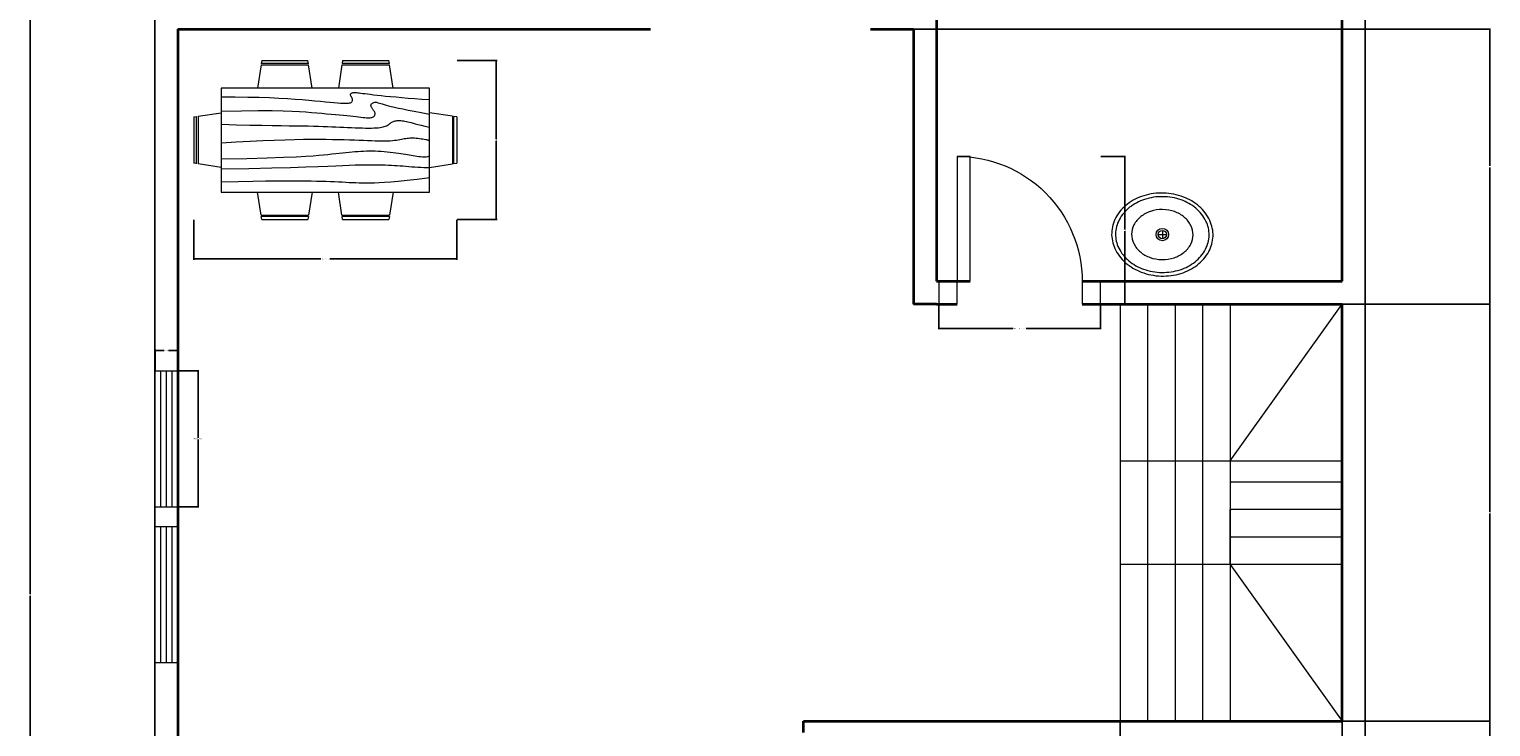
# Model space of a CAD drawing. Units: feet. Extents: x 2306 to 3052, y 829 to 1424.
# Tile 2 of 5: x 2306 to 2625, y 1098 to 1250. Entities that reach past the tile are written whole.
import ezdxf

# ---------------------------------------------------------------- set-up
doc = ezdxf.new("R2010")
doc.units = ezdxf.units.FT
for name, color, linetype, lineweight in [('A-ANNO-DIMS', 2, 'Continuous', 18), ('A-DOOR', 3, 'Continuous', 18), ('A-FLOR-FIXT', 9, 'Continuous', 18), ('A-FLOR-OTLN', 7, 'Continuous', 25), ('A-FLOR-STRS', 7, 'Continuous', 18), ('A-FURN', 8, 'Continuous', 13), ('A-GLAZ', 4, 'Continuous', 18), ('A-WALL', 7, 'Continuous', 35)]:
    doc.layers.add(name, color=color, linetype=linetype, lineweight=lineweight)
doc.styles.get("Standard").update_dxf_attribs({"font": 'arial.ttf'})
doc.dimstyles.get("Standard").update_dxf_attribs({"dimtxt": 0.18, "dimasz": 0.18, "dimexe": 0.18, "dimexo": 0.0625, "dimgap": 0.09, "dimtad": 0, "dimtih": 1, "dimtoh": 1, "dimdec": 4, "dimzin": 0, "dimdsep": 46, "dimlunit": 4, "dimtxsty": 'Standard', "dimcen": 0.09, "dimadec": 0, "dimazin": 0, "dimtfac": 1, "dimtdec": 4, "dimtofl": 0, "dimtmove": 0, "dimatfit": 3, "dimfxl": 1, "dimtolj": 1, "dimtzin": 0, "dimarcsym": 0})

# ---------------------------------------------------------------- blocks, each defined once
blk = doc.blocks.new('Window - Wood Frame 36 in. Wide plan')
for p, q in [((0, 6), (0, 0)), ((0, 4.5), (36, 4.5)), ((36, 6), (36, 0)), ((0, 3), (36, 3)), ((0, 1.5), (36, 1.5))]:
    blk.add_line(p, q)
blk = doc.blocks.new('Dining Set - 36 x 72 in.')
for p, q in [((-22.2343, 26.00059), (-23.4847, 17.99762)), ((-22.2304, 26), (-5.7608, 26)), ((-22, 27.5), (-22.1562, 26.50042)), ((-5.8416, 26.5), (-22.1534, 26.5)), ((-22, 27.5), (-6, 27.5)), ((-5.8437, 26.49966), (-6, 27.5)), ((-4.5152, 17.99762), (-5.7655, 25.99926)), ((5.7657, 26.00059), (4.5153, 17.99762)), ((5.7696, 26), (22.2392, 26)), ((6, 27.5), (5.8438, 26.50042)), ((22.1584, 26.5), (5.8466, 26.5)), ((6, 27.5), (22, 27.5)), ((22.1563, 26.49966), (22, 27.5)), ((23.4848, 17.99762), (22.2345, 25.99926)), ((36, 18), (-36, 18)), ((-36, 18), (-36, -18)), ((36, -18), (36, 18)), ((-45.5, 8), (-44.5004, 8.15617)), ((-45.5, 8), (-45.5, -8)), ((-44.5, -8.15843), (-44.5, 8.15338)), ((-44.0006, 8.23428), (-35.9976, 9.48474)), ((-44, 8.23041), (-44, -8.23915)), ((44.0006, 8.23428), (35.9976, 9.48474)), ((44, 8.23041), (44, -8.23915)), ((44.5, -8.15843), (44.5, 8.15338)), ((45.5, 8), (44.5005, 8.15617)), ((45.5, 8), (45.5, -8)), ((-44.4997, -8.15631), (-45.5, -8)), ((-35.9976, -9.48476), (-43.9993, -8.2345)), ((35.9976, -9.48476), (43.9993, -8.2345)), ((44.4997, -8.15631), (45.5, -8)), ((-36, -18), (36, -18)), ((-22.2343, -26.0006), (-23.4847, -17.99762)), ((-4.5152, -17.99762), (-5.7655, -25.99928)), ((5.7657, -26.0006), (4.5153, -17.99762)), ((23.4848, -17.99762), (22.2345, -25.99928)), ((-22.2304, -26), (-5.7608, -26)), ((-22, -27.5), (-22.1562, -26.50044)), ((-5.8416, -26.5), (-22.1534, -26.5)), ((-22, -27.5), (-6, -27.5)), ((-5.8437, -26.49967), (-6, -27.5)), ((5.7696, -26), (22.2392, -26)), ((6, -27.5), (5.8438, -26.50044)), ((22.1584, -26.5), (5.8466, -26.5)), ((6, -27.5), (22, -27.5)), ((22.1563, -26.49967), (22, -27.5))]:
    blk.add_line(p, q)
for points in [[(-36, 15), (-31.1772, 14.97754), (-26.8079, 14.91406), (-22.8538, 14.81543), (-19.276, 14.6875), (-16.0362, 14.53613), (-13.0957, 14.36718), (-10.4159, 14.18652), (-7.9583, 14), (-5.6904, 13.81315), (-3.6035, 13.63021), (-1.6954, 13.45508), (0.0365, 13.29166), (1.5945, 13.14388), (2.9811, 13.01562), (4.1988, 12.9108), (5.25, 12.83333), (6.1393, 12.78613), (6.8802, 12.76823), (7.4883, 12.77767), (7.9792, 12.8125), (8.3685, 12.87077), (8.6719, 12.95052), (8.9049, 13.0498), (9.0833, 13.16666), (9.2205, 13.29899), (9.3216, 13.44401), (9.3895, 13.59879), (9.4271, 13.76041), (9.4373, 13.92594), (9.4232, 14.09245), (9.3875, 14.257), (9.3333, 14.41666), (9.2638, 14.56917), (9.1836, 14.71484), (9.0975, 14.85465), (9.0104, 14.98958), (8.9272, 15.1206), (8.8529, 15.2487), (8.7922, 15.37483), (8.75, 15.5), (8.7305, 15.62467), (8.7344, 15.74739), (8.7617, 15.86621), (8.8125, 15.97916), (8.8867, 16.08431), (8.9844, 16.17968), (9.1055, 16.26334), (9.25, 16.33333), (9.4189, 16.38802), (9.6172, 16.42708), (9.8506, 16.45052), (10.125, 16.45833), (10.4463, 16.45052), (10.8203, 16.42708), (11.2529, 16.38802), (11.75, 16.33333), (12.3184, 16.26318), (12.9694, 16.17838), (13.7151, 16.07991), (14.5677, 15.96875), (15.5395, 15.84586), (16.6426, 15.71224), (17.8893, 15.56884), (19.2917, 15.41666), (20.859, 15.25667), (22.5879, 15.08984), (24.4721, 14.91715), (26.5052, 14.73958), (28.6809, 14.5581), (30.9929, 14.3737), (33.4347, 14.18733), (36, 14)], [(-36, 10), (-28.9766, 10.14274), (-23.1725, 10.20442), (-18.4241, 10.19775), (-14.5677, 10.13541), (-11.4399, 10.03011), (-8.877, 9.89453), (-6.7154, 9.74137), (-4.7917, 9.58333), (-2.9698, 9.43082), (-1.2246, 9.28515), (0.4415, 9.14534), (2.026, 9.01041), (3.5266, 8.87939), (4.9408, 8.7513), (6.266, 8.62516), (7.5, 8.5), (8.6411, 8.37549), (9.6914, 8.2539), (10.6538, 8.13818), (11.5312, 8.03125), (12.3267, 7.93603), (13.043, 7.85547), (13.6831, 7.79248), (14.25, 7.75), (14.7471, 7.7303), (15.1797, 7.73307), (15.5537, 7.75732), (15.875, 7.80208), (16.1494, 7.86637), (16.3828, 7.94922), (16.5811, 8.04964), (16.75, 8.16666), (16.8944, 8.29915), (17.0143, 8.44531), (17.1089, 8.60319), (17.1771, 8.77083), (17.218, 8.94629), (17.2305, 9.1276), (17.2137, 9.31282), (17.1667, 9.5), (17.0895, 9.6875), (16.987, 9.875), (16.8649, 10.0625), (16.7292, 10.25), (16.5856, 10.4375), (16.4401, 10.625), (16.2985, 10.8125), (16.1667, 11), (16.05, 11.18733), (15.9518, 11.3737), (15.8752, 11.5581), (15.8229, 11.73958), (15.798, 11.91715), (15.8034, 12.08984), (15.842, 12.25667), (15.9167, 12.41666), (16.0295, 12.56836), (16.1784, 12.70833), (16.3605, 12.83268), (16.5729, 12.9375), (16.8127, 13.01888), (17.0768, 13.07291), (17.3625, 13.0957), (17.6667, 13.08333), (17.9894, 13.03312), (18.3418, 12.94726), (18.7382, 12.82918), (19.1927, 12.68229), (19.7195, 12.51001), (20.3327, 12.31575), (21.0465, 12.10294), (21.875, 11.875), (22.8357, 11.63354), (23.959, 11.37304), (25.2786, 11.08618), (26.8282, 10.76562), (28.6414, 10.40405), (30.752, 9.99414), (33.1936, 9.52856), (36, 9)], [(-36, 5.5), (-30.7157, 5.3348), (-26.069, 5.20963), (-21.9946, 5.11767), (-18.4271, 5.05208), (-15.3009, 5.00602), (-12.5508, 4.97265), (-10.1112, 4.94515), (-7.9167, 4.91666), (-5.909, 4.88167), (-4.0586, 4.83984), (-2.3429, 4.79215), (-0.7396, 4.73958), (0.7739, 4.6831), (2.22, 4.6237), (3.6213, 4.56233), (5, 4.5), (6.373, 4.43782), (7.7344, 4.3776), (9.0723, 4.32129), (10.375, 4.27083), (11.6309, 4.22819), (12.8281, 4.19531), (13.9551, 4.17415), (15, 4.16666), (15.954, 4.17448), (16.819, 4.19791), (17.6001, 4.23698), (18.3021, 4.29166), (18.9299, 4.36198), (19.4883, 4.44791), (19.9823, 4.54948), (20.4167, 4.66666), (20.7969, 4.79899), (21.1302, 4.94401), (21.4245, 5.09879), (21.6875, 5.26041), (21.9271, 5.42594), (22.1511, 5.59245), (22.3672, 5.757), (22.5834, 5.91666), (22.8065, 6.06868), (23.0404, 6.21093), (23.2879, 6.34147), (23.5521, 6.45833), (23.8358, 6.55957), (24.142, 6.64323), (24.4735, 6.70735), (24.8334, 6.75), (25.2235, 6.76969), (25.642, 6.76692), (26.0858, 6.74267), (26.5521, 6.69791), (27.0379, 6.63362), (27.5404, 6.55078), (28.0565, 6.45036), (28.5834, 6.33333), (29.1242, 6.19987), (29.7071, 6.04687), (30.3661, 5.87044), (31.1354, 5.66666), (32.0493, 5.43164), (33.142, 5.16146), (34.4475, 4.85221), (36, 4.5)], [(-36, -1), (-30.7915, -0.6591), (-26.0195, -0.38216), (-21.6519, -0.16284), (-17.6563, 0.00521), (-14.0005, 0.12833), (-10.6523, 0.21289), (-7.5796, 0.26522), (-4.75, 0.29166), (-2.134, 0.29793), (0.2878, 0.28711), (2.5317, 0.26163), (4.6146, 0.22396), (6.5529, 0.17651), (8.3633, 0.12174), (10.0623, 0.06209), (11.6667, 0), (13.1899, -0.06201), (14.6341, -0.1211), (15.9982, -0.17432), (17.2813, -0.21875), (18.4823, -0.25147), (19.6003, -0.26953), (20.6343, -0.27002), (21.5834, -0.25), (22.4481, -0.20768), (23.2357, -0.14584), (23.9549, -0.06836), (24.6146, 0.02083), (25.2235, 0.11784), (25.7904, 0.21875), (26.3241, 0.31966), (26.8334, 0.41666), (27.3265, 0.50618), (27.8099, 0.58593), (28.2894, 0.65397), (28.7709, 0.70833), (29.2601, 0.74707), (29.763, 0.76823), (30.2855, 0.76985), (30.8334, 0.75), (31.4088, 0.70784), (31.9994, 0.64713), (32.589, 0.57275), (33.1615, 0.48958), (33.7008, 0.4025), (34.1908, 0.3164), (34.6153, 0.23616), (34.9584, 0.16666), (35.2099, 0.11165), (35.3848, 0.07031), (35.504, 0.04069), (35.5886, 0.02083), (35.6594, 0.00879), (35.7377, 0.0026), (35.8442, 0.00032), (36, 0)], [(-36, -6.5), (-27.1843, -6.31267), (-20.084, -6.1263), (-14.469, -5.9419), (-10.1094, -5.76042), (-6.7752, -5.58285), (-4.2363, -5.41016), (-2.2629, -5.24333), (-0.625, -5.08334), (0.8708, -4.93099), (2.2715, -4.78646), (3.5872, -4.64974), (4.8281, -4.52084), (6.0046, -4.39974), (7.127, -4.28646), (8.2053, -4.18099), (9.25, -4.08334), (10.2705, -3.99382), (11.2734, -3.91407), (12.2647, -3.84603), (13.25, -3.79167), (14.2354, -3.75293), (15.2266, -3.73177), (16.2295, -3.73015), (17.25, -3.75), (18.2912, -3.79248), (19.3451, -3.85547), (20.4009, -3.93604), (21.4479, -4.03125), (22.4754, -4.13819), (23.4727, -4.25391), (24.4289, -4.37549), (25.3334, -4.5), (26.1785, -4.62492), (26.9694, -4.74935), (27.7145, -4.87281), (28.4219, -4.99479), (29.1, -5.11483), (29.7572, -5.23242), (30.4016, -5.34709), (31.0417, -5.45834), (31.6837, -5.56437), (32.3262, -5.65821), (32.9658, -5.73153), (33.599, -5.77604), (34.2224, -5.78345), (34.8327, -5.74545), (35.4264, -5.65373), (36, -5.5)], [(-36, -10), (-26.4022, -9.81299), (-18.4675, -9.62891), (-11.9839, -9.45069), (-6.7396, -9.28125), (-2.5226, -9.12354), (0.8789, -8.98047), (3.6769, -8.85498), (6.0833, -8.75), (8.2767, -8.66765), (10.3021, -8.60677), (12.1712, -8.56543), (13.8958, -8.54167), (15.4876, -8.53353), (16.9583, -8.53907), (18.3197, -8.55632), (19.5834, -8.58334), (20.7616, -8.61841), (21.8685, -8.66081), (22.9188, -8.71004), (23.9271, -8.76563), (24.9081, -8.82707), (25.8763, -8.89388), (26.8465, -8.96558), (27.8334, -9.04167), (28.8474, -9.12118), (29.8828, -9.20117), (30.93, -9.27824), (31.9792, -9.34896), (33.0205, -9.40991), (34.0443, -9.45768), (35.0407, -9.48885), (36, -9.5)], [(-36, -14.5), (-30.0881, -14.33513), (-25.0332, -14.21224), (-20.7312, -14.12647), (-17.0781, -14.07292), (-13.97, -14.04671), (-11.3027, -14.04297), (-8.9724, -14.05681), (-6.875, -14.08334), (-4.9224, -14.11833), (-3.0905, -14.16016), (-1.3709, -14.20785), (0.2448, -14.26042), (1.7647, -14.3169), (3.1973, -14.3763), (4.5507, -14.43767), (5.8333, -14.5), (7.0554, -14.5621), (8.235, -14.62175), (9.3922, -14.67652), (10.5469, -14.72396), (11.7192, -14.76164), (12.929, -14.78711), (14.1965, -14.79794), (15.5417, -14.79167), (16.9933, -14.76424), (18.6152, -14.70508), (20.4804, -14.60197), (22.6615, -14.44271), (25.2312, -14.21509), (28.2624, -13.9069), (31.8277, -13.50594), (36, -13)]]:
    blk.add_lwpolyline(points)
blk = doc.blocks.new('Sink - Oval top')
for p, q in [((-1, 0), (1, 0)), ((0, 1), (0, -1))]:
    blk.add_line(p, q)
for points in [[(-12.23, 0.39, 0.117634), (-11.46, -3.36, 0.104469), (-8.88, -6.8, 0.090016), (-5.08, -9.07, 0.08192), (-0.32, -10.02, 0.08192), (4.49, -9.38, 0.090016), (8.42, -7.36, 0.104469), (11.22, -4.09, 0.117634), (12.23, -0.39, 0.117634), (11.46, 3.36, 0.104469), (8.88, 6.8, 0.090016), (5.08, 9.07, 0.08192), (0.32, 10.02, 0.08192), (-4.49, 9.38, 0.090016), (-8.42, 7.36, 0.104469), (-11.22, 4.09, 0.117634)], [(-11.29, 0.16, 0.118622), (-10.52, -3.25, 0.104678), (-8.07, -6.36, 0.089562), (-4.54, -8.37, 0.081185), (-0.13, -9.15, 0.081185), (4.3, -8.49, 0.089562), (7.89, -6.58, 0.104678), (10.42, -3.55, 0.118622), (11.29, -0.16, 0.118622), (10.52, 3.25, 0.104678), (8.07, 6.36, 0.089562), (4.54, 8.37, 0.081185), (0.13, 9.15, 0.081185), (-4.3, 8.49, 0.089562), (-7.89, 6.58, 0.104678), (-10.42, 3.55, 0.118622)], [(-7.42, 0.08, 0.118283), (-6.91, -2.17, 0.104607), (-5.29, -4.21, 0.089718), (-2.97, -5.53, 0.081436), (-0.07, -6.04, 0.081436), (2.84, -5.59, 0.089718), (5.2, -4.33, 0.104607), (6.86, -2.32, 0.118283), (7.42, -0.08, 0.118283), (6.91, 2.17, 0.104607), (5.29, 4.21, 0.089718), (2.97, 5.53, 0.081436), (0.07, 6.04, 0.081436), (-2.84, 5.59, 0.089718), (-5.2, 4.33, 0.104607), (-6.86, 2.32, 0.118283)]]:
    blk.add_lwpolyline(points, format="xyb", close=True)
for radius in [1.5, 1]:
    blk.add_circle((0, 0), radius)
blk = doc.blocks.new('DOOR-SWING-STANDARD')
blk.add_lwpolyline([(4.02, 32.25), (4.02, 5), (1.75, 5)])
blk.add_lwpolyline([(4.02, 5), (6.86, 5), (6.86, 32.25), (6.29, 32.25), (4.02, 32.25, -0.414214), (31.27, 5)], format="xyb")
for points in [[(0, 5), (0, 0), (4, 0), (4, 5)], [(31.27, 5), (31.27, 0), (35.27, 0), (35.27, 5)]]:
    blk.add_lwpolyline(points, close=True)
blk = doc.blocks.new('*D16')
at = {"layer": 'A-ANNO-DIMS', "color": 0, "lineweight": -2, "transparency": 16777216}
for p, q in [((2338.87, 1175.76), (2343.43, 1175.76)), ((2343.25, 1175.58), (2343.25, 1161.12)), ((2343.25, 1146.3), (2343.25, 1160.76)), ((2338.87, 1146.12), (2343.43, 1146.12))]:
    blk.add_line(p, q, dxfattribs=at)
at = {"layer": 'A-ANNO-DIMS', "color": 0, "transparency": 16777216}
for points in [[(2343.22, 1175.58), (2343.28, 1175.58), (2343.25, 1175.76)], [(2343.22, 1146.3), (2343.28, 1146.3), (2343.25, 1146.12)]]:
    blk.add_solid(points, dxfattribs=at)
at = {"layer": 'Defpoints', "color": 0, "transparency": 16777216}
for p in [(2338.8, 1175.76), (2343.25, 1175.76), (2338.8, 1146.12)]:
    blk.add_point(p, dxfattribs=at)
at = {"layer": 'A-ANNO-DIMS', "color": 0, "transparency": 16777216, "insert": (2343.25, 1160.94), "char_height": 0.18, "attachment_point": 5}
blk.add_mtext('\\A1;WINDOW 30 TYP.', dxfattribs=at)
blk = doc.blocks.new('*D17')
at = {"layer": 'A-ANNO-DIMS', "color": 0, "lineweight": -2, "transparency": 16777216}
for p, q in [((2333.86, 1175.82), (2333.86, 1180.39)), ((2334.04, 1180.21), (2335.87, 1180.21)), ((2338.62, 1180.21), (2336.79, 1180.21)), ((2338.8, 1175.82), (2338.8, 1180.39))]:
    blk.add_line(p, q, dxfattribs=at)
at = {"layer": 'A-ANNO-DIMS', "color": 0, "transparency": 16777216}
for points in [[(2334.04, 1180.24), (2334.04, 1180.18), (2333.86, 1180.21)], [(2338.62, 1180.24), (2338.62, 1180.18), (2338.8, 1180.21)]]:
    blk.add_solid(points, dxfattribs=at)
at = {"layer": 'Defpoints', "color": 0, "transparency": 16777216}
for p in [(2333.86, 1180.21), (2333.86, 1175.76), (2338.8, 1175.76)]:
    blk.add_point(p, dxfattribs=at)
at = {"layer": 'A-ANNO-DIMS', "color": 0, "transparency": 16777216, "insert": (2336.33, 1180.21), "char_height": 0.18, "attachment_point": 5}
blk.add_mtext('\\A1;5 TYP.', dxfattribs=at)
blk = doc.blocks.new('*D20')
at = {"layer": 'A-ANNO-DIMS', "color": 0, "lineweight": -2, "transparency": 16777216}
for p, q in [((2504.8, 1190.26), (2504.8, 1184.86)), ((2540.07, 1190.26), (2540.07, 1184.86)), ((2504.98, 1185.04), (2521, 1185.04)), ((2539.89, 1185.04), (2523.87, 1185.04))]:
    blk.add_line(p, q, dxfattribs=at)
at = {"layer": 'A-ANNO-DIMS', "color": 0, "transparency": 16777216}
for points in [[(2504.98, 1185.07), (2504.98, 1185.01), (2504.8, 1185.04)], [(2539.89, 1185.07), (2539.89, 1185.01), (2540.07, 1185.04)]]:
    blk.add_solid(points, dxfattribs=at)
at = {"layer": 'Defpoints', "color": 0, "transparency": 16777216}
for p in [(2504.8, 1190.33), (2540.07, 1190.33), (2540.07, 1185.04)]:
    blk.add_point(p, dxfattribs=at)
at = {"layer": 'A-ANNO-DIMS', "color": 0, "transparency": 16777216, "insert": (2522.43, 1185.04), "char_height": 0.18, "attachment_point": 5}
blk.add_mtext('\\A1;SINGLE DOOR 35 TYP.', dxfattribs=at)
blk = doc.blocks.new('*D21')
at = {"layer": 'A-ANNO-DIMS', "color": 0, "lineweight": -2, "transparency": 16777216}
for p, q in [((2540.13, 1222.58), (2545.54, 1222.58)), ((2545.36, 1222.4), (2545.36, 1206.64)), ((2545.36, 1190.51), (2545.36, 1206.27)), ((2540.13, 1190.33), (2545.54, 1190.33))]:
    blk.add_line(p, q, dxfattribs=at)
at = {"layer": 'A-ANNO-DIMS', "color": 0, "transparency": 16777216}
for points in [[(2545.33, 1222.4), (2545.39, 1222.4), (2545.36, 1222.58)], [(2545.33, 1190.51), (2545.39, 1190.51), (2545.36, 1190.33)]]:
    blk.add_solid(points, dxfattribs=at)
at = {"layer": 'Defpoints', "color": 0, "transparency": 16777216}
for p in [(2540.07, 1222.58), (2545.36, 1222.58), (2540.07, 1190.33)]:
    blk.add_point(p, dxfattribs=at)
at = {"layer": 'A-ANNO-DIMS', "color": 0, "transparency": 16777216, "insert": (2545.36, 1206.45), "char_height": 0.18, "attachment_point": 5}
blk.add_mtext('\\A1;32 TYP.', dxfattribs=at)
blk = doc.blocks.new('*D38')
at = {"layer": 'A-ANNO-DIMS', "color": 0, "lineweight": -2, "transparency": 16777216}
for p, q in [((2342.3, 1208.72), (2342.3, 1200)), ((2399.69, 1208.72), (2399.69, 1200)), ((2342.48, 1200.18), (2370.03, 1200.18)), ((2399.51, 1200.18), (2371.96, 1200.18))]:
    blk.add_line(p, q, dxfattribs=at)
at = {"layer": 'A-ANNO-DIMS', "color": 0, "transparency": 16777216}
for points in [[(2342.48, 1200.21), (2342.48, 1200.15), (2342.3, 1200.18)], [(2399.51, 1200.21), (2399.51, 1200.15), (2399.69, 1200.18)]]:
    blk.add_solid(points, dxfattribs=at)
at = {"layer": 'Defpoints', "color": 0, "transparency": 16777216}
for p in [(2342.3, 1208.78), (2399.69, 1208.78), (2399.69, 1200.18)]:
    blk.add_point(p, dxfattribs=at)
at = {"layer": 'A-ANNO-DIMS', "color": 0, "transparency": 16777216, "insert": (2371, 1200.18), "char_height": 0.18, "attachment_point": 5}
blk.add_mtext('\\A1;DINING SET 57', dxfattribs=at)
blk = doc.blocks.new('*D39')
at = {"layer": 'A-ANNO-DIMS', "color": 0, "lineweight": -2, "transparency": 16777216}
for p, q in [((2399.75, 1243.47), (2408.47, 1243.47)), ((2408.29, 1243.29), (2408.29, 1226.31)), ((2408.29, 1208.96), (2408.29, 1225.94)), ((2399.75, 1208.78), (2408.47, 1208.78))]:
    blk.add_line(p, q, dxfattribs=at)
at = {"layer": 'A-ANNO-DIMS', "color": 0, "transparency": 16777216}
for points in [[(2408.26, 1243.29), (2408.32, 1243.29), (2408.29, 1243.47)], [(2408.26, 1208.96), (2408.32, 1208.96), (2408.29, 1208.78)]]:
    blk.add_solid(points, dxfattribs=at)
at = {"layer": 'Defpoints', "color": 0, "transparency": 16777216}
for p in [(2399.69, 1243.47), (2408.29, 1243.47), (2399.69, 1208.78)]:
    blk.add_point(p, dxfattribs=at)
at = {"layer": 'A-ANNO-DIMS', "color": 0, "transparency": 16777216, "insert": (2408.29, 1226.13), "char_height": 0.18, "attachment_point": 5}
blk.add_mtext('\\A1;35', dxfattribs=at)
blk = doc.blocks.new('*D47')
at = {"layer": 'A-ANNO-DIMS', "color": 0, "lineweight": -2, "transparency": 16777216}
for p, q in [((2333.74, 1396.83), (2306.45, 1396.83)), ((2306.63, 1396.65), (2306.63, 1127.01)), ((2306.63, 857.01), (2306.63, 1126.65)), ((2333.74, 856.83), (2306.45, 856.83))]:
    blk.add_line(p, q, dxfattribs=at)
at = {"layer": 'A-ANNO-DIMS', "color": 0, "transparency": 16777216}
for points in [[(2306.6, 1396.65), (2306.66, 1396.65), (2306.63, 1396.83)], [(2306.6, 857.01), (2306.66, 857.01), (2306.63, 856.83)]]:
    blk.add_solid(points, dxfattribs=at)
at = {"layer": 'Defpoints', "color": 0, "transparency": 16777216}
for p in [(2306.63, 1396.83), (2333.8, 1396.83), (2333.8, 856.83)]:
    blk.add_point(p, dxfattribs=at)
at = {"layer": 'A-ANNO-DIMS', "color": 0, "transparency": 16777216, "insert": (2306.63, 1126.83), "char_height": 0.18, "attachment_point": 5}
blk.add_mtext('\\A1;540', dxfattribs=at)
blk = doc.blocks.new('*D49')
at = {"layer": 'A-ANNO-DIMS', "color": 0, "lineweight": -2, "transparency": 16777216}
for p, q in [((2592.87, 1099.33), (2625.16, 1099.33)), ((2624.98, 1099.15), (2624.98, 1037.01)), ((2624.98, 974.51), (2624.98, 1036.65)), ((2592.87, 974.33), (2625.16, 974.33))]:
    blk.add_line(p, q, dxfattribs=at)
at = {"layer": 'A-ANNO-DIMS', "color": 0, "transparency": 16777216}
for points in [[(2624.95, 1099.15), (2625.01, 1099.15), (2624.98, 1099.33)], [(2624.95, 974.51), (2625.01, 974.51), (2624.98, 974.33)]]:
    blk.add_solid(points, dxfattribs=at)
at = {"layer": 'Defpoints', "color": 0, "transparency": 16777216}
for p in [(2592.8, 1099.33), (2624.98, 1099.33), (2592.8, 974.33)]:
    blk.add_point(p, dxfattribs=at)
at = {"layer": 'A-ANNO-DIMS', "color": 0, "transparency": 16777216, "insert": (2624.98, 1036.83), "char_height": 0.18, "attachment_point": 5}
blk.add_mtext('\\A1;125', dxfattribs=at)
blk = doc.blocks.new('*D50')
at = {"layer": 'A-ANNO-DIMS', "color": 0, "lineweight": -2, "transparency": 16777216}
for p, q in [((2592.87, 1190.33), (2625.16, 1190.33)), ((2624.98, 1190.15), (2624.98, 1145.01)), ((2624.98, 1099.51), (2624.98, 1144.65)), ((2592.87, 1099.33), (2625.16, 1099.33))]:
    blk.add_line(p, q, dxfattribs=at)
at = {"layer": 'A-ANNO-DIMS', "color": 0, "transparency": 16777216}
for points in [[(2624.95, 1190.15), (2625.01, 1190.15), (2624.98, 1190.33)], [(2624.95, 1099.51), (2625.01, 1099.51), (2624.98, 1099.33)]]:
    blk.add_solid(points, dxfattribs=at)
at = {"layer": 'Defpoints', "color": 0, "transparency": 16777216}
for p in [(2592.8, 1190.33), (2624.98, 1190.33), (2592.8, 1099.33)]:
    blk.add_point(p, dxfattribs=at)
at = {"layer": 'A-ANNO-DIMS', "color": 0, "transparency": 16777216, "insert": (2624.98, 1144.83), "char_height": 0.18, "attachment_point": 5}
blk.add_mtext('\\A1;91', dxfattribs=at)
blk = doc.blocks.new('*D51')
at = {"layer": 'A-ANNO-DIMS', "color": 0, "lineweight": -2, "transparency": 16777216}
for p, q in [((2499.37, 1250.33), (2625.16, 1250.33)), ((2624.98, 1250.15), (2624.98, 1220.51)), ((2624.98, 1190.51), (2624.98, 1220.15)), ((2592.87, 1190.33), (2625.16, 1190.33))]:
    blk.add_line(p, q, dxfattribs=at)
at = {"layer": 'A-ANNO-DIMS', "color": 0, "transparency": 16777216}
for points in [[(2624.95, 1250.15), (2625.01, 1250.15), (2624.98, 1250.33)], [(2624.95, 1190.51), (2625.01, 1190.51), (2624.98, 1190.33)]]:
    blk.add_solid(points, dxfattribs=at)
at = {"layer": 'Defpoints', "color": 0, "transparency": 16777216}
for p in [(2499.3, 1250.33), (2624.98, 1250.33), (2592.8, 1190.33)]:
    blk.add_point(p, dxfattribs=at)
at = {"layer": 'A-ANNO-DIMS', "color": 0, "transparency": 16777216, "insert": (2624.98, 1220.33), "char_height": 0.18, "attachment_point": 5}
blk.add_mtext('\\A1;60', dxfattribs=at)
blk = doc.blocks.new('*D61')
at = {"layer": 'A-ANNO-DIMS', "color": 0, "lineweight": -2, "transparency": 16777216}
for p, q in [((2544.34, 1099.26), (2544.34, 1071.97)), ((2592.8, 1099.26), (2592.8, 1071.97)), ((2544.52, 1072.15), (2568.17, 1072.15)), ((2592.62, 1072.15), (2568.97, 1072.15))]:
    blk.add_line(p, q, dxfattribs=at)
at = {"layer": 'A-ANNO-DIMS', "color": 0, "transparency": 16777216}
for points in [[(2544.52, 1072.18), (2544.52, 1072.12), (2544.34, 1072.15)], [(2592.62, 1072.18), (2592.62, 1072.12), (2592.8, 1072.15)]]:
    blk.add_solid(points, dxfattribs=at)
at = {"layer": 'Defpoints', "color": 0, "transparency": 16777216}
for p in [(2544.34, 1099.33), (2592.8, 1099.33), (2544.34, 1072.15)]:
    blk.add_point(p, dxfattribs=at)
at = {"layer": 'A-ANNO-DIMS', "color": 0, "transparency": 16777216, "insert": (2568.57, 1072.15), "char_height": 0.18, "attachment_point": 5}
blk.add_mtext('\\A1;48.47', dxfattribs=at)

msp = doc.modelspace()

# ---------------------------------------------------------------- linework, layer by layer
at = {"layer": 'A-FLOR-OTLN'}
for p, q in [((2333.803, 1396.827), (2333.803, 856.827)), ((2597.803, 856.827), (2597.803, 1396.827))]:
    msp.add_line(p, q, dxfattribs=at)
at = {"layer": 'A-FLOR-STRS'}
for p, q in [((2544.336, 1190.327), (2544.336, 1099.327)), ((2544.336, 1190.327), (2556.336, 1190.327)), ((2550.336, 1190.327), (2550.336, 1099.327)), ((2556.336, 1190.327), (2556.336, 1099.327)), ((2562.336, 1190.327), (2562.336, 1099.327)), ((2568.336, 1190.327), (2568.336, 1099.327)), ((2568.336, 1156.156), (2592.803, 1190.327)), ((2544.336, 1156.156), (2592.803, 1156.156)), ((2592.803, 1156.156), (2592.803, 1133.499)), ((2568.336, 1151.499), (2568.57, 1151.499)), ((2592.803, 1151.499), (2568.57, 1151.499)), ((2568.336, 1133.499), (2568.336, 1145.499)), ((2568.336, 1145.499), (2568.57, 1145.499)), ((2568.336, 1145.499), (2568.57, 1145.499)), ((2592.803, 1145.499), (2568.57, 1145.499)), ((2592.803, 1145.499), (2568.57, 1145.499)), ((2568.336, 1139.499), (2568.57, 1139.499)), ((2592.803, 1139.499), (2568.57, 1139.499)), ((2592.803, 1133.499), (2544.336, 1133.499)), ((2568.336, 1133.499), (2592.803, 1099.327)), ((2592.803, 1133.499), (2568.57, 1133.499))]:
    msp.add_line(p, q, dxfattribs=at)
at = {"layer": 'A-WALL'}
for p, q in [((2504.303, 1286.327), (2504.303, 1195.327)), ((2592.803, 1195.327), (2592.803, 1286.327)), ((2338.803, 1250.327), (2441.935, 1250.327)), ((2338.803, 1250.327), (2338.803, 979.327)), ((2489.935, 1250.327), (2499.303, 1250.327)), ((2499.303, 1250.327), (2499.303, 1190.327)), ((2504.303, 1195.327), (2511.653, 1195.327)), ((2536.068, 1195.327), (2564.303, 1195.327)), ((2564.303, 1195.327), (2592.803, 1195.327)), ((2504.303, 1190.327), (2499.303, 1190.327)), ((2504.303, 1190.327), (2508.798, 1190.327)), ((2536.068, 1190.327), (2564.303, 1190.327)), ((2564.303, 1190.327), (2592.803, 1190.327)), ((2592.803, 1099.327), (2592.803, 1190.327)), ((2475.303, 1099.327), (2592.803, 1099.327)), ((2475.303, 1096.827), (2475.303, 1099.327))]:
    msp.add_line(p, q, dxfattribs=at)

# ---------------------------------------------------------------- block references
at = {"layer": 'A-DOOR'}
msp.add_blockref('DOOR-SWING-STANDARD', (2504.798, 1190.327), dxfattribs=at)
at = {"layer": 'A-FLOR-FIXT', "xscale": 0.9036611704051442, "yscale": 0.9036611704051442, "zscale": 0.9036611704051442}
msp.add_blockref('Sink - Oval top', (2553.553, 1205.509), dxfattribs=at)
at = {"layer": 'A-FURN', "xscale": 0.6305913735776374, "yscale": 0.6305913735776374, "zscale": 0.6305913735776374}
msp.add_blockref('Dining Set - 36 x 72 in.', (2370.995, 1226.126), dxfattribs=at)
at = {"layer": 'A-GLAZ', "xscale": 0.82338841385576, "yscale": 0.82338841385576, "zscale": 0.82338841385576, "rotation": 90}
for p in [(2338.803, 1146.118), (2338.803, 1112.136)]:
    msp.add_blockref('Window - Wood Frame 36 in. Wide plan', p, dxfattribs=at)

# ---------------------------------------------------------------- dimensions: what is measured, and where the dimension line sits
at = {"layer": 'A-ANNO-DIMS'}
for base, p1, p2, angle, override, picture, middle in [((2306.628, 1396.827), (2333.803, 856.827), (2333.803, 1396.827), 90, {"dimdec": 0, "dimlfac": 1, "dimrnd": 0, "dimzin": 0, "dimdsep": 46, "dimlunit": 2}, '*D47', (2306.628, 1126.827)), ((2624.978, 1250.327), (2592.803, 1190.327), (2499.303, 1250.327), 90, {"dimdec": 0, "dimlfac": 1, "dimrnd": 0, "dimzin": 0, "dimdsep": 46, "dimlunit": 2}, '*D51', (2624.978, 1220.327)), ((2408.295, 1243.467), (2399.687, 1208.785), (2399.687, 1243.467), 90, {"dimdec": 0, "dimlfac": 1, "dimrnd": 0, "dimzin": 0, "dimdsep": 46, "dimlunit": 2}, '*D39', (2408.295, 1226.126)), ((2624.978, 1190.327), (2592.803, 1099.327), (2592.803, 1190.327), 90, {"dimdec": 0, "dimlfac": 1, "dimrnd": 0, "dimzin": 0, "dimdsep": 46, "dimlunit": 2}, '*D50', (2624.978, 1144.827)), ((2544.336, 1072.152), (2592.803, 1099.327), (2544.336, 1099.327), 180, {"dimdec": 2, "dimlfac": 1, "dimrnd": 0, "dimzin": 0, "dimdsep": 46, "dimlunit": 2}, '*D61', (2568.57, 1072.152)), ((2624.978, 1099.327), (2592.803, 974.327), (2592.803, 1099.327), 90, {"dimdec": 0, "dimlfac": 1, "dimrnd": 0, "dimzin": 0, "dimdsep": 46, "dimlunit": 2}, '*D49', (2624.978, 1036.827))]:
    dim = msp.add_linear_dim(base=base, p1=p1, p2=p2, angle=angle, dimstyle='Standard', override=override, dxfattribs=at)
    dim.commit()
    dim.dimension.update_dxf_attribs({"geometry": picture, "text_midpoint": middle})
for base, p1, p2, angle, text, picture, middle in [((2545.359, 1222.581), (2540.068, 1190.327), (2540.068, 1222.581), 90, '<> TYP.', '*D21', (2545.359, 1206.454)), ((2333.863, 1180.206), (2338.803, 1175.759), (2333.863, 1175.759), 180, '<> TYP.', '*D17', (2336.333, 1180.206)), ((2343.25, 1175.759), (2338.803, 1146.118), (2338.803, 1175.759), 90, 'WINDOW <> TYP.', '*D16', (2343.25, 1160.938))]:
    dim = msp.add_linear_dim(base=base, p1=p1, p2=p2, angle=angle, text=text, dimstyle='Standard', override={"dimdec": 0, "dimlfac": 1, "dimrnd": 0, "dimzin": 0, "dimdsep": 46, "dimlunit": 2}, dxfattribs=at)
    dim.commit()
    dim.dimension.update_dxf_attribs({"geometry": picture, "text_midpoint": middle})
for base, p1, p2, text, picture, middle in [((2399.687, 1200.177), (2342.303, 1208.785), (2399.687, 1208.785), 'DINING SET <>', '*D38', (2370.995, 1200.177)), ((2540.068, 1185.037), (2504.798, 1190.327), (2540.068, 1190.327), 'SINGLE DOOR <> TYP.', '*D20', (2522.433, 1185.037))]:
    dim = msp.add_linear_dim(base=base, p1=p1, p2=p2, text=text, dimstyle='Standard', override={"dimdec": 0, "dimlfac": 1, "dimrnd": 0, "dimzin": 0, "dimdsep": 46, "dimlunit": 2}, dxfattribs=at)
    dim.commit()
    dim.dimension.update_dxf_attribs({"geometry": picture, "text_midpoint": middle})

doc.saveas('drawing.dxf')
